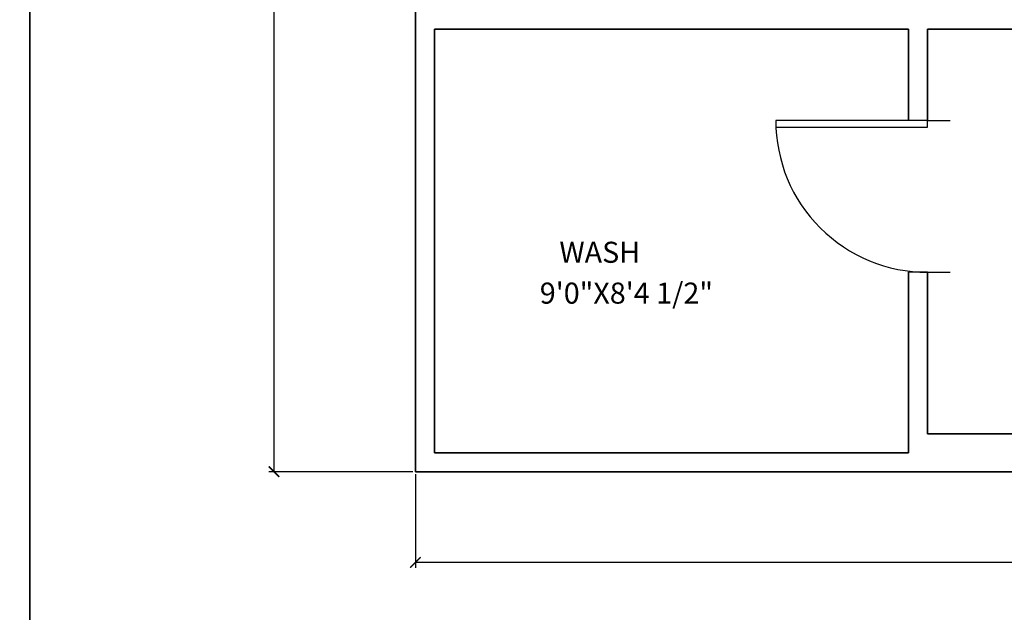
# Model space of a CAD drawing. Units: inches. Extents: x 3283068 to 3284536, y 3240756 to 3241803.
# Tile 3 of 19: x 3283246 to 3283479, y 3241165 to 3241305. Entities that reach past the tile are written whole.
import ezdxf

# ---------------------------------------------------------------- set-up
doc = ezdxf.new("R2010")
doc.units = ezdxf.units.IN
for name, color, linetype, lineweight in [('A-ANNO-DIMS', 2, 'Continuous', 18), ('A-AREA-IDEN', 7, 'Continuous', 18), ('C-PROP', 7, 'Continuous', 25), ('door', 140, 'Continuous', 25), ('wall', 20, 'Continuous', 35)]:
    doc.layers.add(name, color=color, linetype=linetype, lineweight=lineweight)
doc.styles.get("Standard").update_dxf_attribs({"font": 'arial.ttf'})
doc.dimstyles.new('ISO-25', dxfattribs={"dimtxt": 5, "dimasz": 2.5, "dimexe": 1.25, "dimexo": 0.625, "dimtad": 1, "dimlunit": 4, "dimtxsty": 'Standard', "dimblk": 'ARCHTICK', "dimcen": 2.5, "dimadec": 0, "dimazin": 0, "dimtfac": 1, "dimtmove": 0, "dimatfit": 3, "dimfxl": 1, "dimarcsym": 0})

# ---------------------------------------------------------------- blocks, each defined once
blk = doc.blocks.new('_ArchTick')
at = {"color": 0, "linetype": 'ByBlock', "const_width": 0.15}
blk.add_lwpolyline([(-0.5, -0.5), (0.5, 0.5)], dxfattribs=at)
blk = doc.blocks.new('*D1')
at = {"layer": 'A-ANNO-DIMS', "color": 0, "lineweight": -2, "transparency": 16777216}
for p, q in [((3283338.96, 3241639.1), (3283304.8, 3241639.1)), ((3283306.05, 3241198.1), (3283306.05, 3241639.1)), ((3283338.96, 3241198.1), (3283304.8, 3241198.1))]:
    blk.add_line(p, q, dxfattribs=at)
at = {"layer": 'Defpoints', "color": 0, "transparency": 16777216}
for p in [(3283306.05, 3241639.1), (3283339.59, 3241639.1), (3283339.59, 3241198.1)]:
    blk.add_point(p, dxfattribs=at)
at = {"layer": 'A-ANNO-DIMS', "color": 0, "lineweight": -2, "transparency": 16777216, "xscale": 2.5, "yscale": 2.5, "zscale": 2.5}
for p, rotation in [((3283306.05, 3241639.1), 90), ((3283306.05, 3241198.1), 270)]:
    blk.add_blockref('_ArchTick', p, dxfattribs=dict(at, rotation=rotation))
at = {"layer": 'A-ANNO-DIMS', "color": 0, "transparency": 16777216, "insert": (3283302.87, 3241418.6), "char_height": 5, "attachment_point": 5, "rotation": 90}
blk.add_mtext('36\'-9"', dxfattribs=at)
blk = doc.blocks.new('*U7')
for p, q in [((0, 0), (0, 6)), ((40, 0), (40, 6))]:
    blk.add_line(p, q)
blk.add_lwpolyline([(0, 0), (0, -40), (1.75, -40), (1.75, 0)], close=True)
blk.add_arc((0, 0), 40, 270, 0)
blk = doc.blocks.new('*D29')
at = {"layer": 'A-ANNO-DIMS', "color": 0, "lineweight": -2, "transparency": 16777216}
for p, q in [((3283339.59, 3241197.48), (3283339.59, 3241175.31)), ((3283828.59, 3241197.48), (3283828.59, 3241175.31)), ((3283828.59, 3241176.56), (3283339.59, 3241176.56))]:
    blk.add_line(p, q, dxfattribs=at)
at = {"layer": 'Defpoints', "color": 0, "transparency": 16777216}
for p in [(3283339.59, 3241198.1), (3283828.59, 3241198.1), (3283339.59, 3241176.56)]:
    blk.add_point(p, dxfattribs=at)
at = {"layer": 'A-ANNO-DIMS', "color": 0, "lineweight": -2, "transparency": 16777216, "xscale": 2.5, "yscale": 2.5, "zscale": 2.5, "rotation": 180}
blk.add_blockref('_ArchTick', (3283339.59, 3241176.56), dxfattribs=at)
at = {"layer": 'A-ANNO-DIMS', "color": 0, "lineweight": -2, "transparency": 16777216, "xscale": 2.5, "yscale": 2.5, "zscale": 2.5}
blk.add_blockref('_ArchTick', (3283828.59, 3241176.56), dxfattribs=at)
at = {"layer": 'A-ANNO-DIMS', "color": 0, "transparency": 16777216, "insert": (3283584.09, 3241179.74), "char_height": 5, "attachment_point": 5}
blk.add_mtext('40\'-9"', dxfattribs=at)
blk = doc.blocks.new('*D61')
at = {"layer": 'A-ANNO-DIMS', "color": 0, "lineweight": -2, "transparency": 16777216}
for p, q in [((3283247.46, 3241730.6), (3283073.57, 3241730.6)), ((3283074.82, 3241082.6), (3283074.82, 3241730.6)), ((3283247.46, 3241082.6), (3283073.57, 3241082.6))]:
    blk.add_line(p, q, dxfattribs=at)
at = {"layer": 'Defpoints', "color": 0, "transparency": 16777216}
for p in [(3283074.82, 3241730.6), (3283248.09, 3241730.6), (3283248.09, 3241082.6)]:
    blk.add_point(p, dxfattribs=at)
at = {"layer": 'A-ANNO-DIMS', "color": 0, "lineweight": -2, "transparency": 16777216, "xscale": 2.5, "yscale": 2.5, "zscale": 2.5}
for p, rotation in [((3283074.82, 3241730.6), 90), ((3283074.82, 3241082.6), 270)]:
    blk.add_blockref('_ArchTick', p, dxfattribs=dict(at, rotation=rotation))
at = {"layer": 'A-ANNO-DIMS', "color": 0, "transparency": 16777216, "insert": (3283071.64, 3241406.6), "char_height": 5, "attachment_point": 5, "rotation": 90}
blk.add_mtext('54\'-0"', dxfattribs=at)
blk = doc.blocks.new('*D63')
at = {"layer": 'A-ANNO-DIMS', "color": 0, "lineweight": -2, "transparency": 16777216}
for p, q in [((3283248.09, 3241083.23), (3283248.09, 3241798.08)), ((3283248.09, 3241796.83), (3284328.09, 3241796.83)), ((3284328.09, 3241083.23), (3284328.09, 3241798.08))]:
    blk.add_line(p, q, dxfattribs=at)
at = {"layer": 'Defpoints', "color": 0, "transparency": 16777216}
for p in [(3284328.09, 3241796.83), (3283248.09, 3241082.6), (3284328.09, 3241082.6)]:
    blk.add_point(p, dxfattribs=at)
at = {"layer": 'A-ANNO-DIMS', "color": 0, "lineweight": -2, "transparency": 16777216, "xscale": 2.5, "yscale": 2.5, "zscale": 2.5, "rotation": 180}
blk.add_blockref('_ArchTick', (3283248.09, 3241796.83), dxfattribs=at)
at = {"layer": 'A-ANNO-DIMS', "color": 0, "lineweight": -2, "transparency": 16777216, "xscale": 2.5, "yscale": 2.5, "zscale": 2.5}
blk.add_blockref('_ArchTick', (3284328.09, 3241796.83), dxfattribs=at)
at = {"layer": 'A-ANNO-DIMS', "color": 0, "transparency": 16777216, "insert": (3283788.09, 3241800.01), "char_height": 5, "attachment_point": 5}
blk.add_mtext('90\'-0"', dxfattribs=at)

msp = doc.modelspace()

# ---------------------------------------------------------------- linework, layer by layer
at = {"layer": 'C-PROP'}
msp.add_line((3283248.089, 3241730.602), (3283248.089, 3241082.602), dxfattribs=at)
at = {"layer": 'door'}
for p, q in [((3283461.089, 3241281.412), (3283456.589, 3241281.412)), ((3283461.089, 3241245.412), (3283456.589, 3241245.412))]:
    msp.add_line(p, q, dxfattribs=at)
at = {"layer": 'wall'}
for p, q in [((3283339.589, 3241639.102), (3283339.589, 3241198.102)), ((3283344.089, 3241202.602), (3283344.089, 3241303.102)), ((3283348.589, 3241303.102), (3283344.089, 3241303.102)), ((3283348.589, 3241303.102), (3283456.589, 3241303.102)), ((3283456.589, 3241281.412), (3283456.589, 3241303.102)), ((3283461.089, 3241303.102), (3283507.589, 3241303.102)), ((3283461.089, 3241281.412), (3283461.089, 3241303.102)), ((3283456.589, 3241202.602), (3283456.589, 3241245.412)), ((3283461.089, 3241207.102), (3283461.089, 3241245.412)), ((3283461.089, 3241207.102), (3283605.089, 3241207.102)), ((3283348.589, 3241202.602), (3283344.089, 3241202.602)), ((3283348.589, 3241202.602), (3283456.589, 3241202.602)), ((3283339.589, 3241198.102), (3284236.589, 3241198.102))]:
    msp.add_line(p, q, dxfattribs=at)

# ---------------------------------------------------------------- block references
at = {"layer": 'door', "xscale": 0.9, "yscale": 0.9, "zscale": 0.9, "rotation": 270}
msp.add_blockref('*U7', (3283461.089, 3241281.412), dxfattribs=at)

# ---------------------------------------------------------------- texts
at = {"layer": 'A-AREA-IDEN'}
for s, p in [('WASH', (3283373.752, 3241247.663)), ('9\'0"X8\'4 1/2"', (3283369.101, 3241237.97))]:
    msp.add_text(s, height=5, dxfattribs=at).set_placement(p)

# ---------------------------------------------------------------- dimensions: what is measured, and where the dimension line sits
at = {"layer": 'A-ANNO-DIMS'}
for base, p1, p2, override, picture, middle in [((3284328.089, 3241796.827), (3283248.089, 3241082.602), (3284328.089, 3241082.602), {"dimdec": 1, "dimlfac": 1, "dimrnd": 0, "dimzin": 1, "dimdsep": 46, "dimlunit": 4, "dimfrac": 2}, '*D63', (3283788.089, 3241800.005)), ((3283339.589, 3241176.561), (3283828.589, 3241198.102), (3283339.589, 3241198.102), {"dimclrd": 0, "dimclre": 0, "dimclrt": 0}, '*D29', (3283584.089, 3241179.739))]:
    dim = msp.add_linear_dim(base=base, p1=p1, p2=p2, dimstyle='ISO-25', override=override, dxfattribs=at)
    dim.commit()
    dim.dimension.update_dxf_attribs({"geometry": picture, "text_midpoint": middle})
for base, p1, p2, override, picture, middle in [((3283074.817, 3241730.602), (3283248.089, 3241082.602), (3283248.089, 3241730.602), {"dimdec": 1, "dimlfac": 1, "dimrnd": 0, "dimzin": 1, "dimdsep": 46, "dimlunit": 4, "dimfrac": 2}, '*D61', (3283071.639, 3241406.602)), ((3283306.051, 3241639.102), (3283339.589, 3241198.102), (3283339.589, 3241639.102), {"dimclrd": 0, "dimclre": 0, "dimclrt": 0}, '*D1', (3283302.872, 3241418.602))]:
    dim = msp.add_linear_dim(base=base, p1=p1, p2=p2, angle=90, dimstyle='ISO-25', override=override, dxfattribs=at)
    dim.commit()
    dim.dimension.update_dxf_attribs({"geometry": picture, "text_midpoint": middle})

doc.saveas('drawing.dxf')
